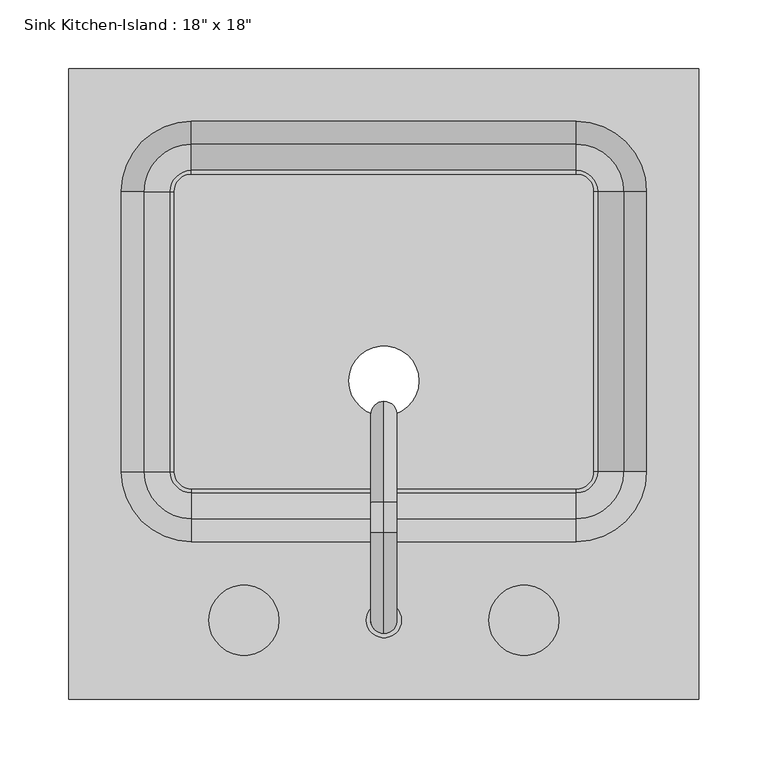
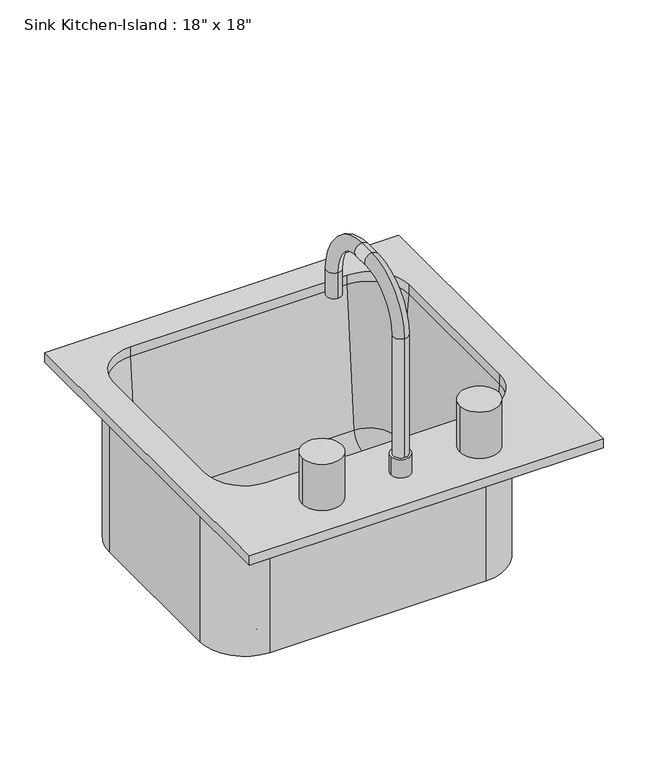
"""IFC4 building model written with IfcOpenShell, lengths in millimetres: flow terminal geometry."""

from ifc_helpers import new_model, si_unit, point, frame, frame_2d, origin, place, context, project, spatial, polyline, circle_curve, ellipse_curve, trimmed, segment, composite_curve, outline, extrude, source, transform, mapped, element, save
from ifc_brep_helpers import plane_surface, cylinder_surface, revolved_surface, advanced_brep


def flow_terminal_41332a36(model_context):
    return source(origin(), model_context, "Body", "SolidModel", [
        advanced_brep(
        [(244.2892406, -230.9454011, 927.1), (244.2892406, 226.2545989, 927.1), (-212.9107594, 226.2545989, 927.1), (-212.9107594, -230.9454011, 927.1), (155.3892406, -116.6454011, 927.1), (-124.0107594, -116.6454011, 927.1), (-174.8107594, -65.8454011, 927.1), (-174.8107594, 137.3545989, 927.1), (-124.0107594, 188.1545989, 927.1), (155.3892406, 188.1545989, 927.1), (206.1892406, 137.3545989, 927.1), (206.1892406, -65.8454011, 927.1), (244.2892406, -230.9454011, 914.4), (-212.9107594, -230.9454011, 914.4), (-212.9107594, 226.2545989, 914.4), (244.2892406, 226.2545989, 914.4), (212.5392406, -65.8454011, 914.4), (212.5392406, 137.3545989, 914.4), (155.3892406, 194.5045989, 914.4), (-124.0107594, 194.5045989, 914.4), (-181.1607594, 137.3545989, 914.4), (-181.1607594, -65.8454011, 914.4), (-124.0107594, -122.9954011, 914.4), (155.3892406, -122.9954011, 914.4), (206.1892406, -65.8454011, 914.4), (155.3892406, -116.6454011, 914.4), (206.1892406, 137.3545989, 914.4), (155.3892406, 188.1545989, 914.4), (-124.0107594, 188.1545989, 914.4), (-174.8107594, 137.3545989, 914.4), (-174.8107594, -65.8454011, 914.4), (-124.0107594, -116.6454011, 914.4), (212.5392406, -65.8454011, 698.5), (155.3892406, -122.9954011, 698.5), (155.3892406, -78.5454011, 698.5), (168.0892406, -65.8454011, 698.5), (155.3892406, -78.5454011, 708.025), (168.0892406, -65.8454011, 708.025), (155.3892406, -81.1338193, 708.025), (170.6776588, -65.8454011, 708.025), (155.3892406, -100.1113283, 725.4146831), (189.6551678, -65.8454011, 725.4146831), (212.5392406, 137.3545989, 698.5), (168.0892406, 137.3545989, 698.5), (168.0892406, 137.3545989, 708.025), (170.6776588, 137.3545989, 708.025), (189.6551678, 137.3545989, 725.4146831), (155.3892406, 194.5045989, 698.5), (155.3892406, 150.0545989, 698.5), (155.3892406, 150.0545989, 708.025), (155.3892406, 152.6430171, 708.025), (155.3892406, 171.6205261, 725.4146831), (-124.0107594, 194.5045989, 698.5), (-124.0107594, 150.0545989, 698.5), (-124.0107594, 150.0545989, 708.025), (-124.0107594, 152.6430171, 708.025), (-124.0107594, 171.6205261, 725.4146831), (-181.1607594, 137.3545989, 698.5), (-136.7107594, 137.3545989, 698.5), (-136.7107594, 137.3545989, 708.025), (-139.2991776, 137.3545989, 708.025), (-158.2766866, 137.3545989, 725.4146831), (-181.1607594, -65.8454011, 698.5), (-136.7107594, -65.8454011, 698.5), (-136.7107594, -65.8454011, 708.025), (-139.2991776, -65.8454011, 708.025), (-158.2766866, -65.8454011, 725.4146831), (-124.0107594, -122.9954011, 698.5), (-124.0107594, -78.5454011, 698.5), (-124.0107594, -78.5454011, 708.025), (-124.0107594, -81.1338193, 708.025), (-124.0107594, -100.1113283, 725.4146831)],
        [
            (0, 1),
            (1, 2),
            (2, 3),
            (3, 0),
            (4, 5),
            (5, 6, circle_curve(frame((-124.0107594, -65.8454011, 927.1), z_axis=(0.0, 0.0, -1.0), x_axis=(1.0, 0.0, 0.0)), 50.8)),
            (6, 7),
            (7, 8, circle_curve(frame((-124.0107594, 137.3545989, 927.1), z_axis=(0.0, 0.0, -1.0), x_axis=(1.0, 0.0, 0.0)), 50.8)),
            (8, 9),
            (9, 10, circle_curve(frame((155.3892406, 137.3545989, 927.1), z_axis=(0.0, 0.0, -1.0), x_axis=(1.0, 0.0, 0.0)), 50.8)),
            (10, 11),
            (11, 4, circle_curve(frame((155.3892406, -65.8454011, 927.1), z_axis=(0.0, 0.0, -1.0), x_axis=(1.0, 0.0, 0.0)), 50.8)),
            (12, 13),
            (13, 14),
            (14, 15),
            (15, 12),
            (16, 17),
            (17, 18, circle_curve(frame((155.3892406, 137.3545989, 914.4), z_axis=(0.0, 0.0, 1.0), x_axis=(1.0, 0.0, 0.0)), 57.15)),
            (18, 19),
            (19, 20, circle_curve(frame((-124.0107594, 137.3545989, 914.4), z_axis=(0.0, 0.0, 1.0), x_axis=(0.0, 1.0, 0.0)), 57.15)),
            (20, 21),
            (21, 22, circle_curve(frame((-124.0107594, -65.8454011, 914.4), z_axis=(0.0, 0.0, 1.0), x_axis=(-1.0, 0.0, 0.0)), 57.15)),
            (22, 23),
            (23, 16, circle_curve(frame((155.3892406, -65.8454011, 914.4), z_axis=(0.0, 0.0, 1.0), x_axis=(0.0, -1.0, 0.0)), 57.15)),
            (3, 13),
            (12, 0),
            (2, 14),
            (1, 15),
            (11, 24),
            (24, 25, circle_curve(frame((155.3892406, -65.8454011, 914.4), z_axis=(0.0, 0.0, -1.0), x_axis=(1.0, 0.0, 0.0)), 50.8)),
            (25, 4),
            (10, 26),
            (26, 24),
            (9, 27),
            (27, 26, circle_curve(frame((155.3892406, 137.3545989, 914.4), z_axis=(0.0, 0.0, -1.0), x_axis=(1.0, 0.0, 0.0)), 50.8)),
            (8, 28),
            (28, 27),
            (7, 29),
            (29, 28, circle_curve(frame((-124.0107594, 137.3545989, 914.4), z_axis=(0.0, 0.0, -1.0), x_axis=(1.0, 0.0, 0.0)), 50.8)),
            (6, 30),
            (30, 29),
            (5, 31),
            (31, 30, circle_curve(frame((-124.0107594, -65.8454011, 914.4), z_axis=(0.0, 0.0, -1.0), x_axis=(1.0, 0.0, 0.0)), 50.8)),
            (25, 31),
            (32, 16),
            (23, 33),
            (33, 32, circle_curve(frame((155.3892406, -65.8454011, 698.5), z_axis=(0.0, 0.0, 1.0), x_axis=(0.0, -1.0, 0.0)), 57.15)),
            (33, 34),
            (34, 35, circle_curve(frame((155.3892406, -65.8454011, 698.5), z_axis=(0.0, 0.0, 1.0), x_axis=(0.0, -1.0, 0.0)), 12.7)),
            (35, 32),
            (34, 36),
            (36, 37, circle_curve(frame((155.3892406, -65.8454011, 708.025), z_axis=(0.0, 0.0, 1.0), x_axis=(0.0, -1.0, 0.0)), 12.7)),
            (37, 35),
            (36, 38),
            (38, 39, circle_curve(frame((155.3892406, -65.8454011, 708.025), z_axis=(0.0, 0.0, 1.0), x_axis=(0.0, -1.0, 0.0)), 15.2884182)),
            (39, 37),
            (38, 40, circle_curve(frame((155.3892406, -81.1338193, 727.075), z_axis=(-1.0, 0.0, 0.0), x_axis=(0.0, -1.0, 0.0)), 19.05)),
            (40, 41, circle_curve(frame((155.3892406, -65.8454011, 725.4146831), z_axis=(0.0, 0.0, 1.0), x_axis=(0.0, -1.0, 0.0)), 34.2659272)),
            (41, 39, circle_curve(frame((170.6776588, -65.8454011, 727.075), z_axis=(0.0, 1.0, 0.0), x_axis=(1.0, 0.0, 0.0)), 19.05)),
            (40, 25),
            (24, 41),
            (32, 42),
            (42, 17),
            (35, 43),
            (43, 42),
            (37, 44),
            (44, 43),
            (39, 45),
            (45, 44),
            (41, 46),
            (46, 45, circle_curve(frame((170.6776588, 137.3545989, 727.075), z_axis=(0.0, 1.0, 0.0), x_axis=(1.0, 0.0, 0.0)), 19.05)),
            (26, 46),
            (42, 47, circle_curve(frame((155.3892406, 137.3545989, 698.5), z_axis=(0.0, 0.0, 1.0), x_axis=(1.0, 0.0, 0.0)), 57.15)),
            (47, 18),
            (43, 48, circle_curve(frame((155.3892406, 137.3545989, 698.5), z_axis=(0.0, 0.0, 1.0), x_axis=(1.0, 0.0, 0.0)), 12.7)),
            (48, 47),
            (44, 49, circle_curve(frame((155.3892406, 137.3545989, 708.025), z_axis=(0.0, 0.0, 1.0), x_axis=(1.0, 0.0, 0.0)), 12.7)),
            (49, 48),
            (45, 50, circle_curve(frame((155.3892406, 137.3545989, 708.025), z_axis=(0.0, 0.0, 1.0), x_axis=(1.0, 0.0, 0.0)), 15.2884182)),
            (50, 49),
            (46, 51, circle_curve(frame((155.3892406, 137.3545989, 725.4146831), z_axis=(0.0, 0.0, 1.0), x_axis=(1.0, 0.0, 0.0)), 34.2659272)),
            (51, 50, circle_curve(frame((155.3892406, 152.6430171, 727.075), z_axis=(-1.0, 0.0, 0.0), x_axis=(0.0, 1.0, 0.0)), 19.05)),
            (27, 51),
            (47, 52),
            (52, 19),
            (48, 53),
            (53, 52),
            (49, 54),
            (54, 53),
            (50, 55),
            (55, 54),
            (51, 56),
            (56, 55, circle_curve(frame((-124.0107594, 152.6430171, 727.075), z_axis=(-1.0, 0.0, 0.0), x_axis=(0.0, 1.0, 0.0)), 19.05)),
            (28, 56),
            (52, 57, circle_curve(frame((-124.0107594, 137.3545989, 698.5), z_axis=(0.0, 0.0, 1.0), x_axis=(0.0, 1.0, 0.0)), 57.15)),
            (57, 20),
            (53, 58, circle_curve(frame((-124.0107594, 137.3545989, 698.5), z_axis=(0.0, 0.0, 1.0), x_axis=(0.0, 1.0, 0.0)), 12.7)),
            (58, 57),
            (54, 59, circle_curve(frame((-124.0107594, 137.3545989, 708.025), z_axis=(0.0, 0.0, 1.0), x_axis=(0.0, 1.0, 0.0)), 12.7)),
            (59, 58),
            (55, 60, circle_curve(frame((-124.0107594, 137.3545989, 708.025), z_axis=(0.0, 0.0, 1.0), x_axis=(0.0, 1.0, 0.0)), 15.2884182)),
            (60, 59),
            (56, 61, circle_curve(frame((-124.0107594, 137.3545989, 725.4146831), z_axis=(0.0, 0.0, 1.0), x_axis=(0.0, 1.0, 0.0)), 34.2659272)),
            (61, 60, circle_curve(frame((-139.2991776, 137.3545989, 727.075), z_axis=(0.0, -1.0, 0.0), x_axis=(-1.0, 0.0, 0.0)), 19.05)),
            (29, 61),
            (57, 62),
            (62, 21),
            (58, 63),
            (63, 62),
            (59, 64),
            (64, 63),
            (60, 65),
            (65, 64),
            (61, 66),
            (66, 65, circle_curve(frame((-139.2991776, -65.8454011, 727.075), z_axis=(0.0, -1.0, 0.0), x_axis=(-1.0, 0.0, 0.0)), 19.05)),
            (30, 66),
            (62, 67, circle_curve(frame((-124.0107594, -65.8454011, 698.5), z_axis=(0.0, 0.0, 1.0), x_axis=(-1.0, 0.0, 0.0)), 57.15)),
            (67, 22),
            (63, 68, circle_curve(frame((-124.0107594, -65.8454011, 698.5), z_axis=(0.0, 0.0, 1.0), x_axis=(-1.0, 0.0, 0.0)), 12.7)),
            (68, 67),
            (64, 69, circle_curve(frame((-124.0107594, -65.8454011, 708.025), z_axis=(0.0, 0.0, 1.0), x_axis=(-1.0, 0.0, 0.0)), 12.7)),
            (69, 68),
            (65, 70, circle_curve(frame((-124.0107594, -65.8454011, 708.025), z_axis=(0.0, 0.0, 1.0), x_axis=(-1.0, 0.0, 0.0)), 15.2884182)),
            (70, 69),
            (66, 71, circle_curve(frame((-124.0107594, -65.8454011, 725.4146831), z_axis=(0.0, 0.0, 1.0), x_axis=(-1.0, 0.0, 0.0)), 34.2659272)),
            (71, 70, circle_curve(frame((-124.0107594, -81.1338193, 727.075), z_axis=(1.0, 0.0, 0.0), x_axis=(0.0, -1.0, 0.0)), 19.05)),
            (31, 71),
            (67, 33),
            (68, 34),
            (69, 36),
            (70, 38),
            (71, 40),
        ],
        [
            plane_surface(frame((-212.9107594, -230.9454011, 927.1), z_axis=(0.0, 0.0, 1.0), x_axis=(-1.0, 0.0, 0.0))),
            plane_surface(frame((-212.9107594, -230.9454011, 914.4), z_axis=(0.0, 0.0, -1.0), x_axis=(1.0, 0.0, 0.0))),
            plane_surface(frame((244.2892406, -230.9454011, 927.1), z_axis=(0.0, -1.0, 0.0), x_axis=(0.0, 0.0, -1.0))),
            plane_surface(frame((-212.9107594, -230.9454011, 927.1), z_axis=(-1.0, 0.0, 0.0), x_axis=(0.0, 0.0, -1.0))),
            plane_surface(frame((-212.9107594, 226.2545989, 927.1), z_axis=(0.0, 1.0, 0.0), x_axis=(0.0, 0.0, -1.0))),
            plane_surface(frame((244.2892406, 226.2545989, 927.1), z_axis=(1.0, 0.0, 0.0), x_axis=(0.0, 0.0, -1.0))),
            revolved_surface(polyline([(206.1892406, -65.8454011, 914.4), (206.1892406, -65.8454011, 927.1)]), (155.3892406, -65.8454011, 0.0), (0.0, 0.0, -1.0)),
            plane_surface(frame((206.1892406, -65.8454011, 927.1), z_axis=(-1.0, 0.0, 0.0), x_axis=(0.0, 0.0, -1.0))),
            revolved_surface(polyline([(206.1892406, 137.3545989, 914.4), (206.1892406, 137.3545989, 927.1)]), (155.3892406, 137.3545989, 0.0), (0.0, 0.0, -1.0)),
            plane_surface(frame((155.3892406, 188.1545989, 927.1), z_axis=(0.0, -1.0, 0.0), x_axis=(0.0, 0.0, -1.0))),
            revolved_surface(polyline([(-73.2107594, 137.3545989, 914.4), (-73.2107594, 137.3545989, 927.1)]), (-124.0107594, 137.3545989, 0.0), (0.0, 0.0, -1.0)),
            plane_surface(frame((-174.8107594, 137.3545989, 927.1), z_axis=(1.0, 0.0, 0.0), x_axis=(0.0, 0.0, -1.0))),
            revolved_surface(polyline([(-73.2107594, -65.8454011, 914.4), (-73.2107594, -65.8454011, 927.1)]), (-124.0107594, -65.8454011, 0.0), (0.0, 0.0, -1.0)),
            plane_surface(frame((-124.0107594, -116.6454011, 927.1), z_axis=(0.0, 1.0, 0.0), x_axis=(0.0, 0.0, -1.0))),
            cylinder_surface(frame((155.3892406, -65.8454011, 0.0), z_axis=(0.0, 0.0, -1.0), x_axis=(0.0, -1.0, 0.0)), 57.15),
            plane_surface(frame((155.3892406, -65.8454011, 698.5), z_axis=(0.0, 0.0, -1.0), x_axis=(0.0, -1.0, 0.0))),
            revolved_surface(polyline([(155.3892406, -78.5454011, 698.5), (155.3892406, -78.5454011, 708.025)]), (155.3892406, -65.8454011, 0.0), (0.0, 0.0, -1.0)),
            plane_surface(frame((155.3892406, -65.8454011, 708.025), z_axis=(0.0, 0.0, 1.0), x_axis=(0.0, -1.0, 0.0))),
            revolved_surface(trimmed(ellipse_curve(frame((155.3892406, -81.1338193, 727.075), z_axis=(-1.0, 0.0, 0.0), x_axis=(0.0, -1.0, 0.0)), 19.05, 19.05), [point((155.3892406, -81.1338193, 708.025))], [point((155.3892406, -100.1113283, 725.4146831))], True, "CARTESIAN"), (155.3892406, -65.8454011, 0.0), (0.0, 0.0, -1.0)),
            revolved_surface(polyline([(155.3892406, -100.1113283, 725.4146831), (155.3892406, -116.6454011, 914.4)]), (155.3892406, -65.8454011, 0.0), (0.0, 0.0, -1.0)),
            plane_surface(frame((212.5392406, -65.8454011, 914.4), z_axis=(1.0, 0.0, 0.0), x_axis=(0.0, 1.0, 0.0))),
            plane_surface(frame((212.5392406, -65.8454011, 698.5), z_axis=(0.0, 0.0, -1.0), x_axis=(0.0, 1.0, 0.0))),
            plane_surface(frame((168.0892406, -65.8454011, 698.5), z_axis=(-1.0, 0.0, 0.0), x_axis=(0.0, 1.0, 0.0))),
            plane_surface(frame((168.0892406, -65.8454011, 708.025), z_axis=(0.0, 0.0, 1.0), x_axis=(0.0, 1.0, 0.0))),
            revolved_surface(polyline([(189.7276588, 137.3545989, 727.075), (189.7276588, -65.8454011, 727.075)]), (170.6776588, -65.8454011, 727.075), (0.0, 1.0, 0.0)),
            plane_surface(frame((189.6551678, -65.8454011, 725.4146831), z_axis=(-0.9961946980917443, 0.0, 0.08715574274767254), x_axis=(0.0, 1.0, 0.0))),
            cylinder_surface(frame((155.3892406, 137.3545989, 0.0), z_axis=(0.0, 0.0, -1.0), x_axis=(1.0, 0.0, 0.0)), 57.15),
            plane_surface(frame((155.3892406, 137.3545989, 698.5), z_axis=(0.0, 0.0, -1.0), x_axis=(1.0, 0.0, 0.0))),
            revolved_surface(polyline([(168.08924059999998, 137.3545989, 698.5), (168.08924059999998, 137.3545989, 708.025)]), (155.3892406, 137.3545989, 0.0), (0.0, 0.0, -1.0)),
            plane_surface(frame((155.3892406, 137.3545989, 708.025), z_axis=(0.0, 0.0, 1.0), x_axis=(1.0, 0.0, 0.0))),
            revolved_surface(trimmed(ellipse_curve(frame((170.6776588, 137.3545989, 727.075), z_axis=(0.0, -1.0, 0.0), x_axis=(1.0, 0.0, 0.0)), 19.05, 19.05), [point((170.6776588, 137.3545989, 708.025))], [point((189.6551678, 137.3545989, 725.4146831))], True, "CARTESIAN"), (155.3892406, 137.3545989, 0.0), (0.0, 0.0, -1.0)),
            revolved_surface(polyline([(189.6551678, 137.3545989, 725.4146831), (206.1892406, 137.3545989, 914.4)]), (155.3892406, 137.3545989, 0.0), (0.0, 0.0, -1.0)),
            plane_surface(frame((155.3892406, 194.5045989, 914.4), z_axis=(0.0, 1.0, 0.0), x_axis=(-1.0, 0.0, 0.0))),
            plane_surface(frame((155.3892406, 194.5045989, 698.5), z_axis=(0.0, 0.0, -1.0), x_axis=(-1.0, 0.0, 0.0))),
            plane_surface(frame((155.3892406, 150.0545989, 698.5), z_axis=(0.0, -1.0, 0.0), x_axis=(-1.0, 0.0, 0.0))),
            plane_surface(frame((155.3892406, 150.0545989, 708.025), z_axis=(0.0, 0.0, 1.0), x_axis=(-1.0, 0.0, 0.0))),
            revolved_surface(polyline([(-124.01075939999998, 171.69301710000002, 727.075), (155.3892406, 171.69301710000002, 727.075)]), (155.3892406, 152.6430171, 727.075), (-1.0, 0.0, 0.0)),
            plane_surface(frame((155.3892406, 171.6205261, 725.4146831), z_axis=(0.0, -0.9961946980917443, 0.08715574274767254), x_axis=(-1.0, 0.0, 0.0))),
            cylinder_surface(frame((-124.0107594, 137.3545989, 0.0), z_axis=(0.0, 0.0, -1.0), x_axis=(0.0, 1.0, 0.0)), 57.15),
            plane_surface(frame((-124.0107594, 137.3545989, 698.5), z_axis=(0.0, 0.0, -1.0), x_axis=(0.0, 1.0, 0.0))),
            revolved_surface(polyline([(-124.0107594, 150.0545989, 698.5), (-124.0107594, 150.0545989, 708.025)]), (-124.0107594, 137.3545989, 0.0), (0.0, 0.0, -1.0)),
            plane_surface(frame((-124.0107594, 137.3545989, 708.025), z_axis=(0.0, 0.0, 1.0), x_axis=(0.0, 1.0, 0.0))),
            revolved_surface(trimmed(ellipse_curve(frame((-124.0107594, 152.6430171, 727.075), z_axis=(1.0, 0.0, 0.0), x_axis=(0.0, 1.0, 0.0)), 19.05, 19.05), [point((-124.0107594, 152.6430171, 708.025))], [point((-124.0107594, 171.6205261, 725.4146831))], True, "CARTESIAN"), (-124.0107594, 137.3545989, 0.0), (0.0, 0.0, -1.0)),
            revolved_surface(polyline([(-124.0107594, 171.6205261, 725.4146831), (-124.0107594, 188.1545989, 914.4)]), (-124.0107594, 137.3545989, 0.0), (0.0, 0.0, -1.0)),
            plane_surface(frame((-181.1607594, 137.3545989, 914.4), z_axis=(-1.0, 0.0, 0.0), x_axis=(0.0, -1.0, 0.0))),
            plane_surface(frame((-181.1607594, 137.3545989, 698.5), z_axis=(0.0, 0.0, -1.0), x_axis=(0.0, -1.0, 0.0))),
            plane_surface(frame((-136.7107594, 137.3545989, 698.5), z_axis=(1.0, 0.0, 0.0), x_axis=(0.0, -1.0, 0.0))),
            plane_surface(frame((-136.7107594, 137.3545989, 708.025), z_axis=(0.0, 0.0, 1.0), x_axis=(0.0, -1.0, 0.0))),
            revolved_surface(polyline([(-158.34917760000002, -65.8454011, 727.075), (-158.34917760000002, 137.3545989, 727.075)]), (-139.2991776, 137.3545989, 727.075), (0.0, -1.0, 0.0)),
            plane_surface(frame((-158.2766866, 137.3545989, 725.4146831), z_axis=(0.9961946980917443, 0.0, 0.08715574274767254), x_axis=(0.0, -1.0, 0.0))),
            cylinder_surface(frame((-124.0107594, -65.8454011, 0.0), z_axis=(0.0, 0.0, -1.0), x_axis=(-1.0, 0.0, 0.0)), 57.15),
            plane_surface(frame((-124.0107594, -65.8454011, 698.5), z_axis=(0.0, 0.0, -1.0), x_axis=(-1.0, 0.0, 0.0))),
            revolved_surface(polyline([(-136.7107594, -65.8454011, 698.5), (-136.7107594, -65.8454011, 708.025)]), (-124.0107594, -65.8454011, 0.0), (0.0, 0.0, -1.0)),
            plane_surface(frame((-124.0107594, -65.8454011, 708.025), z_axis=(0.0, 0.0, 1.0), x_axis=(-1.0, 0.0, 0.0))),
            revolved_surface(trimmed(ellipse_curve(frame((-139.2991776, -65.8454011, 727.075), z_axis=(0.0, 1.0, 0.0), x_axis=(-1.0, 0.0, 0.0)), 19.05, 19.05), [point((-139.2991776, -65.8454011, 708.025))], [point((-158.2766866, -65.8454011, 725.4146831))], True, "CARTESIAN"), (-124.0107594, -65.8454011, 0.0), (0.0, 0.0, -1.0)),
            revolved_surface(polyline([(-158.2766866, -65.8454011, 725.4146831), (-174.8107594, -65.8454011, 914.4)]), (-124.0107594, -65.8454011, 0.0), (0.0, 0.0, -1.0)),
            plane_surface(frame((-124.0107594, -122.9954011, 914.4), z_axis=(0.0, -1.0, 0.0), x_axis=(1.0, 0.0, 0.0))),
            plane_surface(frame((-124.0107594, -122.9954011, 698.5), z_axis=(0.0, 0.0, -1.0), x_axis=(1.0, 0.0, 0.0))),
            plane_surface(frame((-124.0107594, -78.5454011, 698.5), z_axis=(0.0, 1.0, 0.0), x_axis=(1.0, 0.0, 0.0))),
            plane_surface(frame((-124.0107594, -78.5454011, 708.025), z_axis=(0.0, 0.0, 1.0), x_axis=(1.0, 0.0, 0.0))),
            revolved_surface(polyline([(155.3892406, -100.1838193, 727.075), (-124.0107594, -100.1838193, 727.075)]), (-124.0107594, -81.1338193, 727.075), (1.0, 0.0, 0.0)),
            plane_surface(frame((-124.0107594, -100.1113283, 725.4146831), z_axis=(0.0, 0.9961946980917443, 0.08715574274767254), x_axis=(1.0, 0.0, 0.0))),
        ],
        [
            (0, [[1, 2, 3, 4], [5, 6, 7, 8, 9, 10, 11, 12]]),
            (1, [[13, 14, 15, 16], [17, 18, 19, 20, 21, 22, 23, 24]]),
            (2, [[25, -13, 26, -4]]),
            (3, [[27, -14, -25, -3]]),
            (4, [[28, -15, -27, -2]]),
            (5, [[-26, -16, -28, -1]]),
            (6, [[29, 30, 31, -12]]),
            (7, [[32, 33, -29, -11]]),
            (8, [[34, 35, -32, -10]]),
            (9, [[36, 37, -34, -9]]),
            (10, [[38, 39, -36, -8]]),
            (11, [[40, 41, -38, -7]]),
            (12, [[42, 43, -40, -6]]),
            (13, [[-31, 44, -42, -5]]),
            (14, [[45, -24, 46, 47]]),
            (15, [[48, 49, 50, -47]]),
            (16, [[51, 52, 53, -49]]),
            (17, [[54, 55, 56, -52]]),
            (18, [[57, 58, 59, -55]]),
            (19, [[60, -30, 61, -58]]),
            (20, [[62, 63, -17, -45]]),
            (21, [[64, 65, -62, -50]]),
            (22, [[66, 67, -64, -53]]),
            (23, [[68, 69, -66, -56]]),
            (24, [[70, 71, -68, -59]]),
            (25, [[-33, 72, -70, -61]]),
            (26, [[73, 74, -18, -63]]),
            (27, [[75, 76, -73, -65]]),
            (28, [[77, 78, -75, -67]]),
            (29, [[79, 80, -77, -69]]),
            (30, [[81, 82, -79, -71]]),
            (31, [[-35, 83, -81, -72]]),
            (32, [[84, 85, -19, -74]]),
            (33, [[86, 87, -84, -76]]),
            (34, [[88, 89, -86, -78]]),
            (35, [[90, 91, -88, -80]]),
            (36, [[92, 93, -90, -82]]),
            (37, [[-37, 94, -92, -83]]),
            (38, [[95, 96, -20, -85]]),
            (39, [[97, 98, -95, -87]]),
            (40, [[99, 100, -97, -89]]),
            (41, [[101, 102, -99, -91]]),
            (42, [[103, 104, -101, -93]]),
            (43, [[-39, 105, -103, -94]]),
            (44, [[106, 107, -21, -96]]),
            (45, [[108, 109, -106, -98]]),
            (46, [[110, 111, -108, -100]]),
            (47, [[112, 113, -110, -102]]),
            (48, [[114, 115, -112, -104]]),
            (49, [[-41, 116, -114, -105]]),
            (50, [[117, 118, -22, -107]]),
            (51, [[119, 120, -117, -109]]),
            (52, [[121, 122, -119, -111]]),
            (53, [[123, 124, -121, -113]]),
            (54, [[125, 126, -123, -115]]),
            (55, [[-43, 127, -125, -116]]),
            (56, [[-23, -118, 128, -46]]),
            (57, [[-128, -120, 129, -48]]),
            (58, [[-129, -122, 130, -51]]),
            (59, [[-130, -124, 131, -54]]),
            (60, [[-131, -126, 132, -57]]),
            (61, [[-132, -127, -44, -60]]),
        ],
    ),
        advanced_brep(
        [(2.9892406, -173.7954011, 927.1), (28.3892406, -173.7954011, 927.1), (15.6892406, -183.3204011, 1114.425), (15.6892406, -183.3204011, 952.5), (15.6892406, -164.2704011, 952.5), (15.6892406, -164.2704011, 1114.425), (15.6892406, -110.2954011, 1168.4), (15.6892406, -110.2954011, 1187.45), (15.6892406, -88.0704011, 1168.4), (15.6892406, -88.0704011, 1187.45), (15.6892406, -34.0954011, 1114.425), (15.6892406, -15.0454011, 1114.425), (15.6892406, -15.0454011, 1079.5), (15.6892406, -34.0954011, 1079.5), (2.9892406, -173.7954011, 952.5), (28.3892406, -173.7954011, 952.5)],
        [
            (0, 1, circle_curve(frame((15.6892406, -173.7954011, 927.1), z_axis=(0.0, 0.0, -1.0), x_axis=(1.0, 0.0, 0.0)), 12.7)),
            (1, 0, circle_curve(frame((15.6892406, -173.7954011, 927.1), z_axis=(0.0, 0.0, -1.0), x_axis=(1.0, 0.0, 0.0)), 12.7)),
            (2, 3),
            (3, 4, circle_curve(frame((15.6892406, -173.7954011, 952.5), z_axis=(0.0, 0.0, 1.0), x_axis=(0.0, 1.0, 0.0)), 9.525)),
            (4, 5),
            (5, 2, circle_curve(frame((15.6892406, -173.7954011, 1114.425), z_axis=(0.0, 0.0, -1.0), x_axis=(0.0, 1.0, 0.0)), 9.525)),
            (4, 3, circle_curve(frame((15.6892406, -173.7954011, 952.5), z_axis=(0.0, 0.0, 1.0), x_axis=(0.0, 1.0, 0.0)), 9.525)),
            (2, 5, circle_curve(frame((15.6892406, -173.7954011, 1114.425), z_axis=(0.0, 0.0, -1.0), x_axis=(0.0, 1.0, 0.0)), 9.525)),
            (5, 6, circle_curve(frame((15.6892406, -110.2954011, 1114.425), z_axis=(-1.0, 0.0, 0.0), x_axis=(0.0, -1.0, 0.0)), 53.975)),
            (6, 7, circle_curve(frame((15.6892406, -110.2954011, 1177.925), z_axis=(0.0, -1.0, 0.0), x_axis=(0.0, 0.0, -1.0)), 9.525)),
            (7, 2, circle_curve(frame((15.6892406, -110.2954011, 1114.425), z_axis=(1.0, 0.0, 0.0), x_axis=(0.0, -1.0, 0.0)), 73.025)),
            (7, 6, circle_curve(frame((15.6892406, -110.2954011, 1177.925), z_axis=(0.0, -1.0, 0.0), x_axis=(0.0, 0.0, -1.0)), 9.525)),
            (6, 8),
            (8, 9, circle_curve(frame((15.6892406, -88.0704011, 1177.925), z_axis=(0.0, -1.0, 0.0), x_axis=(0.0, 0.0, -1.0)), 9.525)),
            (9, 7),
            (9, 8, circle_curve(frame((15.6892406, -88.0704011, 1177.925), z_axis=(0.0, -1.0, 0.0), x_axis=(0.0, 0.0, -1.0)), 9.525)),
            (8, 10, circle_curve(frame((15.6892406, -88.0704011, 1114.425), z_axis=(-1.0, 0.0, 0.0), x_axis=(0.0, 0.0, 1.0)), 53.975)),
            (10, 11, circle_curve(frame((15.6892406, -24.5704011, 1114.425), z_axis=(0.0, 0.0, 1.0), x_axis=(0.0, -1.0, 0.0)), 9.525)),
            (11, 9, circle_curve(frame((15.6892406, -88.0704011, 1114.425), z_axis=(1.0, 0.0, 0.0), x_axis=(0.0, 0.0, 1.0)), 73.025)),
            (11, 10, circle_curve(frame((15.6892406, -24.5704011, 1114.425), z_axis=(0.0, 0.0, 1.0), x_axis=(0.0, -1.0, 0.0)), 9.525)),
            (12, 13, circle_curve(frame((15.6892406, -24.5704011, 1079.5), z_axis=(0.0, 0.0, -1.0), x_axis=(0.0, -1.0, 0.0)), 9.525)),
            (13, 12, circle_curve(frame((15.6892406, -24.5704011, 1079.5), z_axis=(0.0, 0.0, -1.0), x_axis=(0.0, -1.0, 0.0)), 9.525)),
            (10, 13),
            (12, 11),
            (14, 15, circle_curve(frame((15.6892406, -173.7954011, 952.5), z_axis=(0.0, 0.0, 1.0), x_axis=(1.0, 0.0, 0.0)), 12.7)),
            (15, 14, circle_curve(frame((15.6892406, -173.7954011, 952.5), z_axis=(0.0, 0.0, 1.0), x_axis=(1.0, 0.0, 0.0)), 12.7)),
            (15, 1),
            (0, 14),
        ],
        [
            plane_surface(frame((15.6892406, -164.2704011, 927.1), z_axis=(0.0, 0.0, -1.0), x_axis=(1.0, 0.0, 0.0))),
            cylinder_surface(frame((15.6892406, -173.7954011, 927.1), z_axis=(0.0, 0.0, -1.0), x_axis=(0.0, 1.0, 0.0)), 9.525),
            revolved_surface(trimmed(ellipse_curve(frame((15.6892406, -173.7954011, 1114.425), z_axis=(0.0, 0.0, 1.0), x_axis=(0.0, 1.0, 0.0)), 9.525, 9.525), [point((15.6892406, -183.3204011, 1114.425))], [point((15.6892406, -164.2704011, 1114.425))], True, "CARTESIAN"), (15.6892406, -110.2954011, 1114.425), (1.0, 0.0, 0.0)),
            revolved_surface(trimmed(ellipse_curve(frame((15.6892406, -173.7954011, 1114.425), z_axis=(0.0, 0.0, 1.0), x_axis=(0.0, 1.0, 0.0)), 9.525, 9.525), [point((15.6892406, -164.2704011, 1114.425))], [point((15.6892406, -183.3204011, 1114.425))], True, "CARTESIAN"), (15.6892406, -110.2954011, 1114.425), (1.0, 0.0, 0.0)),
            cylinder_surface(frame((15.6892406, -110.2954011, 1177.925), z_axis=(0.0, -1.0, 0.0), x_axis=(0.0, 0.0, -1.0)), 9.525),
            revolved_surface(trimmed(ellipse_curve(frame((15.6892406, -88.0704011, 1177.925), z_axis=(0.0, 1.0, 0.0), x_axis=(0.0, 0.0, -1.0)), 9.525, 9.525), [point((15.6892406, -88.0704011, 1187.45))], [point((15.6892406, -88.0704011, 1168.4))], True, "CARTESIAN"), (15.6892406, -88.0704011, 1114.425), (1.0, 0.0, 0.0)),
            revolved_surface(trimmed(ellipse_curve(frame((15.6892406, -88.0704011, 1177.925), z_axis=(0.0, 1.0, 0.0), x_axis=(0.0, 0.0, -1.0)), 9.525, 9.525), [point((15.6892406, -88.0704011, 1168.4))], [point((15.6892406, -88.0704011, 1187.45))], True, "CARTESIAN"), (15.6892406, -88.0704011, 1114.425), (1.0, 0.0, 0.0)),
            plane_surface(frame((15.6892406, -15.0454011, 1079.5), z_axis=(0.0, 0.0, -1.0), x_axis=(-1.0, 0.0, 0.0))),
            cylinder_surface(frame((15.6892406, -24.5704011, 1114.425), z_axis=(0.0, 0.0, 1.0), x_axis=(0.0, -1.0, 0.0)), 9.525),
            plane_surface(frame((28.3892406, -173.7954011, 952.5), z_axis=(0.0, 0.0, 1.0), x_axis=(0.0, -1.0, 0.0))),
            cylinder_surface(frame((15.6892406, -173.7954011, 927.1), z_axis=(0.0, 0.0, 1.0), x_axis=(1.0, 0.0, 0.0)), 12.7),
        ],
        [
            (0, [[1, 2]]),
            (1, [[3, 4, 5, 6]]),
            (1, [[-5, 7, -3, 8]]),
            (2, [[9, 10, 11, -6]]),
            (3, [[-11, 12, -9, -8]]),
            (4, [[13, 14, 15, -10]]),
            (4, [[-15, 16, -13, -12]]),
            (5, [[17, 18, 19, -14]]),
            (6, [[-19, 20, -17, -16]]),
            (7, [[21, 22]]),
            (8, [[23, -21, 24, -18]]),
            (8, [[-24, -22, -23, -20]]),
            (9, [[25, 26], [-7, -4]]),
            (10, [[27, -1, 28, -26]]),
            (10, [[-28, -2, -27, -25]]),
        ],
    ),
        extrude(outline(composite_curve([segment(trimmed(circle_curve(frame_2d((-85.9107594, -173.7954011)), 25.4), [point((-111.3107594, -173.7954011))], [point((-60.5107594, -173.7954011))], False, "CARTESIAN"), True, "CONTINUOUS"), segment(trimmed(circle_curve(frame_2d((-85.9107594, -173.7954011)), 25.4), [point((-60.5107594, -173.7954011))], [point((-111.3107594, -173.7954011))], False, "CARTESIAN"), True, "CONTINUOUS")], self_intersect=False)), frame((0.0, 0.0, 927.1), z_axis=(0.0, 0.0, 1.0), x_axis=(1.0, 0.0, 0.0)), (0.0, 0.0, 1.0), 63.5),
        extrude(outline(composite_curve([segment(trimmed(circle_curve(frame_2d((117.2892406, -173.7954011)), 25.4), [point((91.8892406, -173.7954011))], [point((142.6892406, -173.7954011))], False, "CARTESIAN"), True, "CONTINUOUS"), segment(trimmed(circle_curve(frame_2d((117.2892406, -173.7954011)), 25.4), [point((142.6892406, -173.7954011))], [point((91.8892406, -173.7954011))], False, "CARTESIAN"), True, "CONTINUOUS")], self_intersect=False)), frame((0.0, 0.0, 927.1), z_axis=(0.0, 0.0, 1.0), x_axis=(1.0, 0.0, 0.0)), (0.0, 0.0, 1.0), 63.5),
        extrude(outline(composite_curve([segment(polyline([(155.3892406, -78.5454011), (-124.0107594, -78.5454011)]), True, "CONTINUOUS"), segment(trimmed(circle_curve(frame_2d((-124.0107594, -65.8454011)), 12.7), [point((-124.0107594, -78.5454011))], [point((-136.7107594, -65.8454011))], False, "CARTESIAN"), True, "CONTINUOUS"), segment(polyline([(-136.7107594, -65.8454011), (-136.7107594, 137.3545989)]), True, "CONTINUOUS"), segment(trimmed(circle_curve(frame_2d((-124.0107594, 137.3545989)), 12.7), [point((-136.7107594, 137.3545989))], [point((-124.0107594, 150.0545989))], False, "CARTESIAN"), True, "CONTINUOUS"), segment(polyline([(-124.0107594, 150.0545989), (155.3892406, 150.0545989)]), True, "CONTINUOUS"), segment(trimmed(circle_curve(frame_2d((155.3892406, 137.3545989)), 12.7), [point((155.3892406, 150.0545989))], [point((168.0892406, 137.3545989))], False, "CARTESIAN"), True, "CONTINUOUS"), segment(polyline([(168.0892406, 137.3545989), (168.0892406, -65.8454011)]), True, "CONTINUOUS"), segment(trimmed(circle_curve(frame_2d((155.3892406, -65.8454011)), 12.7), [point((168.0892406, -65.8454011))], [point((155.3892406, -78.5454011))], False, "CARTESIAN"), True, "CONTINUOUS")], self_intersect=False), holes=[composite_curve([segment(trimmed(circle_curve(frame_2d((15.6892406, 0.0)), 25.4), [point((-9.7107594, 0.0))], [point((41.0892406, 0.0))], True, "CARTESIAN"), True, "CONTINUOUS"), segment(trimmed(circle_curve(frame_2d((15.6892406, 0.0)), 25.4), [point((41.0892406, 0.0))], [point((-9.7107594, 0.0))], True, "CARTESIAN"), True, "CONTINUOUS")], self_intersect=False)]), frame((0.0, 0.0, 698.5), z_axis=(0.0, 0.0, 1.0), x_axis=(1.0, 0.0, 0.0)), (0.0, 0.0, 1.0), 9.525),
    ])


if __name__ == "__main__":
    model = new_model("IFC4")
    model_context = context("Model", 3, world=origin())
    ifc_project = project(units=[si_unit("LENGTHUNIT", "METRE", prefix="MILLI")], contexts=[model_context])
    site = spatial("IfcSite", under=ifc_project)
    building = spatial("IfcBuilding", under=site)
    placement = place(None, origin())
    flow_terminal_shape = flow_terminal_41332a36(model_context)
    element("IfcFlowTerminal", 1, ObjectType="Sink Kitchen-Island : 18\" x 18\"", at=placement, inside=building, context=model_context, shape_type="MappedRepresentation", body=[
        mapped(flow_terminal_shape, transform((0.0, 0.0, 0.0), x_axis=(1.0, 0.0, 0.0), y_axis=(0.0, 1.0, 0.0), z_axis=(0.0, 0.0, 1.0))),
    ])
    save(model, "model.ifc")

# Revit data of these elements
# Type "Sink Kitchen-Island : 18\" x 18\""
#   Assembly Code = "D2010410"
#   Counter Height = 3' - 0"
#   Depth = 1' - 6"
#   Width = 1' - 6"
#   Faucet Material = Steel, Polished
#   Sink Material = Steel, Polished
#   Default Elevation = 0
# Element 1 (IfcFlowTerminal, "Sink Kitchen-Island : 18\" x 18\"")
#   Materials on its faces: "Steel, Polished"
# Materials
#   "Steel, Polished": class "Metal", colour RGB 57 57 57, transparency 0, Description = "Polished steel", Cost = 0
